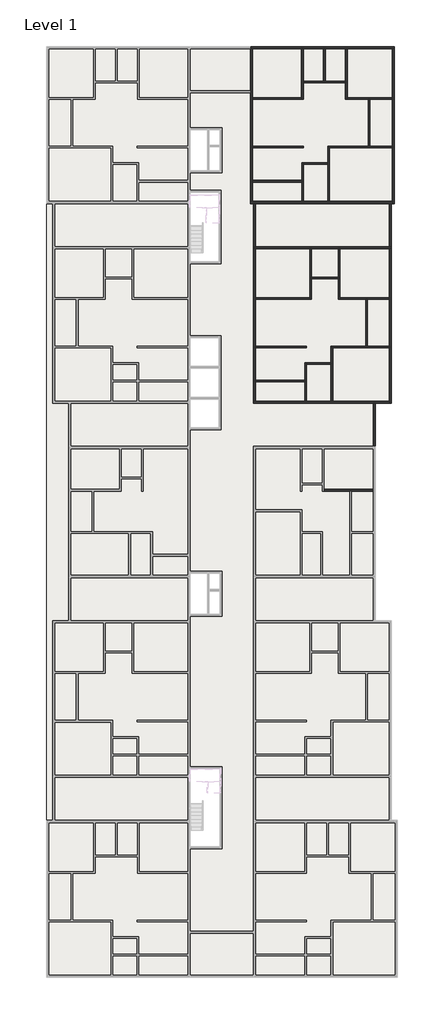
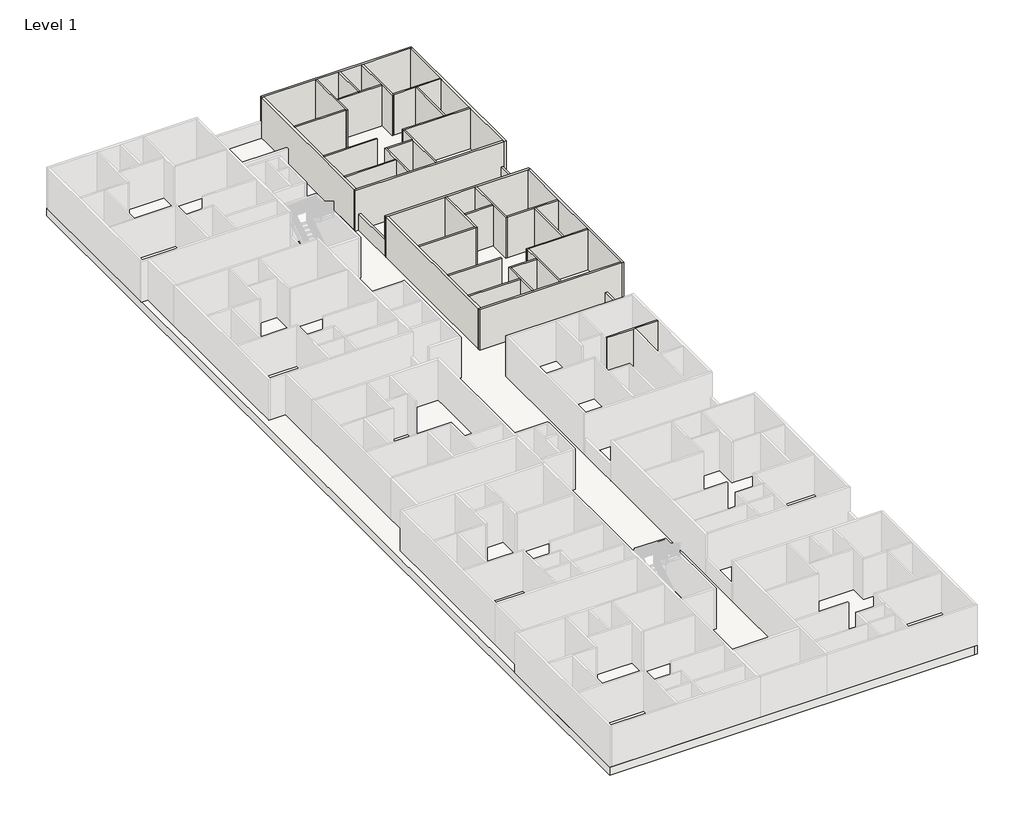
# One storey, part 4 of 8: 37 walls, 1 slab.
"""IFC4 building model written with IfcOpenShell, lengths in millimetres."""

from ifc_helpers import new_model, si_unit, frame, origin, place, context, project, spatial, polyline, outline, extrude, faceted_brep, element, save

model = new_model("IFC4")

# Units and contexts
model_context = context("Model", 3, world=origin())
ifc_project = project(units=[si_unit("LENGTHUNIT", "METRE", prefix="MILLI")], contexts=[model_context])

# Site, building, storey
site = spatial("IfcSite", under=ifc_project)
building = spatial("IfcBuilding", under=site)
storey = spatial("IfcBuildingStorey", under=building, Name="Level 1", Elevation=25234.6172466)

# Slab
placement = place(None, origin())
element("IfcSlab", 1, ObjectType="FLOOR", at=placement, inside=storey, context=model_context, shape_type="SweptSolid", body=[
    extrude(outline(polyline([(-14323.5415084, 35183.5216096), (11584.5443719, 35183.5216096), (11584.5443719, 23499.5216096), (11360.9214687, 23499.5216096), (11360.9214687, 8615.1216096), (10173.4714687, 8615.1216096), (10173.4714687, -7538.7344126), (11360.9214687, -7538.7344126), (11360.9214687, -22423.1344126), (11813.0584916, -22423.1344126), (11813.0584916, -34107.1344126), (11584.5443719, -34107.1344126), (-14323.5415084, -34107.1344126), (-14323.5415084, 35183.5216096)]), holes=[polyline([(-3617.4415084, 29152.4900967), (-3617.4415084, 25799.6900967), (-1255.2415084, 25799.6900967), (-1255.2415084, 29152.4900967), (-3617.4415084, 29152.4900967)]), polyline([(-3617.4415084, 24490.1216096), (-3617.4415084, 19003.7216096), (-1331.4415084, 19003.7216096), (-1331.4415084, 24490.1216096), (-3617.4415084, 24490.1216096)]), polyline([(-3617.4415084, 13669.6303368), (-3617.4415084, 6659.2303368), (-1331.4415084, 6659.2303368), (-1331.4415084, 13669.6303368), (-3617.4415084, 13669.6303368)]), polyline([(-3617.4415084, -3882.2751812), (-3617.4415084, -7235.0751812), (-1255.2415084, -7235.0751812), (-1255.2415084, -3882.2751812), (-3617.4415084, -3882.2751812)]), polyline([(-3617.4415084, -18429.9851539), (-3617.4415084, -24525.9851539), (-1229.8415084, -24525.9851539), (-1229.8415084, -18429.9851539), (-3617.4415084, -18429.9851539)])]), frame((0.0, 0.0, 24625.0172466), z_axis=(0.0, 0.0, 1.0), x_axis=(1.0, 0.0, 0.0)), (0.0, 0.0, 1.0), 609.6),
])

# Walls
element("IfcWall", 2, ObjectType="4.5\"", at=placement, inside=storey, context=model_context, shape_type="Brep", body=[
    faceted_brep([(6363.4714687, 2100.0216096, 25234.6172466), (8282.4584916, 2100.0216096, 25234.6172466), (8396.7584916, 2100.0216096, 25234.6172466), (10021.0714687, 2100.0216096, 25234.6172466), (10021.0714687, 2100.0216096, 28282.6172466), (8396.7584916, 2100.0216096, 28282.6172466), (8282.4584916, 2100.0216096, 28282.6172466), (6363.4714687, 2100.0216096, 28282.6172466), (6363.4714687, 2214.3216096, 25234.6172466), (6363.4714687, 2214.3216096, 28282.6172466), (10021.0714687, 2214.3216096, 28282.6172466), (10021.0714687, 2214.3216096, 25234.6172466)], [[[0, 1, 2, 3, 4, 5, 6, 7]], [[8, 9, 10, 11]], [[3, 2, 1, 0, 8, 11]], [[0, 7, 9, 8]], [[4, 3, 11, 10]], [[7, 6, 5, 4, 10, 9]]]),
])
element("IfcWall", 3, ObjectType="4.5\"", at=placement, inside=storey, context=model_context, shape_type="Brep", body=[
    faceted_brep([(5315.7214687, 20146.7216096, 25234.6172466), (5315.7214687, 16489.1216096, 25234.6172466), (5315.7214687, 16374.8216096, 25234.6172466), (5315.7214687, 16374.8216096, 28282.6172466), (5315.7214687, 16489.1216096, 28282.6172466), (5315.7214687, 20146.7216096, 28282.6172466), (5430.0214687, 20146.7216096, 25234.6172466), (5430.0214687, 20146.7216096, 28282.6172466), (5430.0214687, 18013.1216096, 28282.6172466), (5430.0214687, 17898.8216096, 28282.6172466), (5430.0214687, 16374.8216096, 28282.6172466), (5430.0214687, 16374.8216096, 25234.6172466), (5430.0214687, 17898.8216096, 25234.6172466), (5430.0214687, 18013.1216096, 25234.6172466)], [[[0, 1, 2, 3, 4, 5]], [[6, 7, 8, 9, 10, 11, 12, 13]], [[2, 1, 0, 6, 13, 12, 11]], [[0, 5, 7, 6]], [[3, 2, 11, 10]], [[5, 4, 3, 10, 9, 8, 7]]]),
])
element("IfcWall", 4, ObjectType="4.5\"", at=placement, inside=storey, context=model_context, shape_type="SweptSolid", body=[
    extrude(outline(polyline([(1259.3584916, 16489.1216096), (5315.7214687, 16489.1216096), (5315.7214687, 16374.8216096), (1259.3584916, 16374.8216096), (1259.3584916, 16489.1216096)])), frame((0.0, 0.0, 25234.6172466), z_axis=(0.0, 0.0, 1.0), x_axis=(1.0, 0.0, 0.0)), (0.0, 0.0, 1.0), 3048.0),
])
element("IfcWall", 5, ObjectType="4.5\"", at=placement, inside=storey, context=model_context, shape_type="SweptSolid", body=[
    extrude(outline(polyline([(7436.6214687, 17898.8216096), (5430.0214687, 17898.8216096), (5430.0214687, 18013.1216096), (7436.6214687, 18013.1216096), (7436.6214687, 17898.8216096)])), frame((0.0, 0.0, 25234.6172466), z_axis=(0.0, 0.0, 1.0), x_axis=(1.0, 0.0, 0.0)), (0.0, 0.0, 1.0), 3048.0),
])
element("IfcWall", 6, ObjectType="4.5\"", at=placement, inside=storey, context=model_context, shape_type="Brep", body=[
    faceted_brep([(7436.6214687, 20146.7216096, 25234.6172466), (7436.6214687, 18013.1216096, 25234.6172466), (7436.6214687, 17898.8216096, 25234.6172466), (7436.6214687, 16374.8216096, 25234.6172466), (7436.6214687, 16374.8216096, 28282.6172466), (7436.6214687, 17898.8216096, 28282.6172466), (7436.6214687, 18013.1216096, 28282.6172466), (7436.6214687, 20146.7216096, 28282.6172466), (7550.9214687, 20146.7216096, 25234.6172466), (7550.9214687, 20146.7216096, 28282.6172466), (7550.9214687, 16489.1216096, 28282.6172466), (7550.9214687, 16374.8216096, 28282.6172466), (7550.9214687, 16374.8216096, 25234.6172466), (7550.9214687, 16489.1216096, 25234.6172466)], [[[0, 1, 2, 3, 4, 5, 6, 7]], [[8, 9, 10, 11, 12, 13]], [[3, 2, 1, 0, 8, 13, 12]], [[0, 7, 9, 8]], [[4, 3, 12, 11]], [[7, 6, 5, 4, 11, 10, 9]]]),
])
element("IfcWall", 7, ObjectType="4.5\"", at=placement, inside=storey, context=model_context, shape_type="Brep", body=[
    faceted_brep([(7550.9214687, 16374.8216096, 25234.6172466), (9469.9084916, 16374.8216096, 25234.6172466), (9584.2084916, 16374.8216096, 25234.6172466), (11208.5214687, 16374.8216096, 25234.6172466), (11208.5214687, 16374.8216096, 28282.6172466), (9584.2084916, 16374.8216096, 28282.6172466), (9469.9084916, 16374.8216096, 28282.6172466), (7550.9214687, 16374.8216096, 28282.6172466), (7550.9214687, 16489.1216096, 25234.6172466), (7550.9214687, 16489.1216096, 28282.6172466), (11208.5214687, 16489.1216096, 28282.6172466), (11208.5214687, 16489.1216096, 25234.6172466)], [[[0, 1, 2, 3, 4, 5, 6, 7]], [[8, 9, 10, 11]], [[3, 2, 1, 0, 8, 11]], [[0, 7, 9, 8]], [[4, 3, 11, 10]], [[7, 6, 5, 4, 10, 9]]]),
])
element("IfcWall", 8, ObjectType="4.5\"", at=placement, inside=storey, context=model_context, shape_type="SweptSolid", body=[
    extrude(outline(polyline([(9469.9084916, 12869.6216096), (9469.9084916, 16374.8216096), (9584.2084916, 16374.8216096), (9584.2084916, 12869.6216096), (9469.9084916, 12869.6216096)])), frame((0.0, 0.0, 25234.6172466), z_axis=(0.0, 0.0, 1.0), x_axis=(1.0, 0.0, 0.0)), (0.0, 0.0, 1.0), 3048.0),
])
element("IfcWall", 9, ObjectType="4.5\"", at=placement, inside=storey, context=model_context, shape_type="Brep", body=[
    faceted_brep([(11208.5214687, 12869.6216096, 25234.6172466), (9584.2084916, 12869.6216096, 25234.6172466), (9469.9084916, 12869.6216096, 25234.6172466), (6885.4584916, 12869.6216096, 25234.6172466), (6885.4584916, 12869.6216096, 28282.6172466), (9469.9084916, 12869.6216096, 28282.6172466), (9584.2084916, 12869.6216096, 28282.6172466), (11208.5214687, 12869.6216096, 28282.6172466), (11208.5214687, 12755.3216096, 25234.6172466), (11208.5214687, 12755.3216096, 28282.6172466), (6999.7584916, 12755.3216096, 28282.6172466), (6885.4584916, 12755.3216096, 28282.6172466), (6885.4584916, 12755.3216096, 25234.6172466), (6999.7584916, 12755.3216096, 25234.6172466)], [[[0, 1, 2, 3, 4, 5, 6, 7]], [[8, 9, 10, 11, 12, 13]], [[3, 2, 1, 0, 8, 13, 12]], [[0, 7, 9, 8]], [[4, 3, 12, 11]], [[7, 6, 5, 4, 11, 10, 9]]]),
])
element("IfcWall", 10, ObjectType="4.5\"", at=placement, inside=storey, context=model_context, shape_type="Brep", body=[
    faceted_brep([(6885.4584916, 12755.3216096, 25234.6172466), (6885.4584916, 11663.1216096, 25234.6172466), (6885.4584916, 11548.8216096, 25234.6172466), (6885.4584916, 8767.5216096, 25234.6172466), (6885.4584916, 8767.5216096, 28282.6172466), (6885.4584916, 11548.8216096, 28282.6172466), (6885.4584916, 11663.1216096, 28282.6172466), (6885.4584916, 12755.3216096, 28282.6172466), (6999.7584916, 12755.3216096, 25234.6172466), (6999.7584916, 12755.3216096, 28282.6172466), (6999.7584916, 8767.5216096, 28282.6172466), (6999.7584916, 8767.5216096, 25234.6172466)], [[[0, 1, 2, 3, 4, 5, 6, 7]], [[8, 9, 10, 11]], [[3, 2, 1, 0, 8, 11]], [[0, 7, 9, 8]], [[4, 3, 11, 10]], [[7, 6, 5, 4, 10, 9]]]),
])
element("IfcWall", 11, ObjectType="4.5\"", at=placement, inside=storey, context=model_context, shape_type="Brep", body=[
    faceted_brep([(5056.6584916, 8767.5216096, 25234.6172466), (5056.6584916, 11548.8216096, 25234.6172466), (5056.6584916, 11663.1216096, 25234.6172466), (5056.6584916, 11663.1216096, 28282.6172466), (5056.6584916, 11548.8216096, 28282.6172466), (5056.6584916, 8767.5216096, 28282.6172466), (4942.3584916, 8767.5216096, 25234.6172466), (4942.3584916, 8767.5216096, 28282.6172466), (4942.3584916, 10215.3216096, 28282.6172466), (4942.3584916, 10329.6216096, 28282.6172466), (4942.3584916, 11663.1216096, 28282.6172466), (4942.3584916, 11663.1216096, 25234.6172466), (4942.3584916, 10329.6216096, 25234.6172466), (4942.3584916, 10215.3216096, 25234.6172466)], [[[0, 1, 2, 3, 4, 5]], [[6, 7, 8, 9, 10, 11, 12, 13]], [[2, 1, 0, 6, 13, 12, 11]], [[0, 5, 7, 6]], [[3, 2, 11, 10]], [[5, 4, 3, 10, 9, 8, 7]]]),
])
element("IfcWall", 12, ObjectType="4.5\"", at=placement, inside=storey, context=model_context, shape_type="SweptSolid", body=[
    extrude(outline(polyline([(6885.4584916, 11548.8216096), (5056.6584916, 11548.8216096), (5056.6584916, 11663.1216096), (6885.4584916, 11663.1216096), (6885.4584916, 11548.8216096)])), frame((0.0, 0.0, 25234.6172466), z_axis=(0.0, 0.0, 1.0), x_axis=(1.0, 0.0, 0.0)), (0.0, 0.0, 1.0), 3048.0),
])
element("IfcWall", 13, ObjectType="4.5\"", at=placement, inside=storey, context=model_context, shape_type="SweptSolid", body=[
    extrude(outline(polyline([(4942.3584916, 10215.3216096), (1259.3584916, 10215.3216096), (1259.3584916, 10329.6216096), (4942.3584916, 10329.6216096), (4942.3584916, 10215.3216096)])), frame((0.0, 0.0, 25234.6172466), z_axis=(0.0, 0.0, 1.0), x_axis=(1.0, 0.0, 0.0)), (0.0, 0.0, 1.0), 3048.0),
])
element("IfcWall", 14, ObjectType="4.5\"", at=placement, inside=storey, context=model_context, shape_type="SweptSolid", body=[
    extrude(outline(polyline([(5056.6584916, 12755.3216096), (1259.3584916, 12755.3216096), (1259.3584916, 12869.6216096), (5056.6584916, 12869.6216096), (5056.6584916, 12755.3216096)])), frame((0.0, 0.0, 25234.6172466), z_axis=(0.0, 0.0, 1.0), x_axis=(1.0, 0.0, 0.0)), (0.0, 0.0, 1.0), 3048.0),
])
element("IfcWall", 15, ObjectType="4.5\"", at=placement, inside=storey, context=model_context, shape_type="Brep", body=[
    faceted_brep([(4688.4443719, 35031.1216096, 25234.6172466), (4688.4443719, 31373.5216096, 25234.6172466), (4688.4443719, 31259.2216096, 25234.6172466), (4688.4443719, 31259.2216096, 28282.6172466), (4688.4443719, 31373.5216096, 28282.6172466), (4688.4443719, 35031.1216096, 28282.6172466), (4802.7443719, 35031.1216096, 25234.6172466), (4802.7443719, 35031.1216096, 28282.6172466), (4802.7443719, 32592.7216096, 28282.6172466), (4802.7443719, 32478.4216096, 28282.6172466), (4802.7443719, 31259.2216096, 28282.6172466), (4802.7443719, 31259.2216096, 25234.6172466), (4802.7443719, 32478.4216096, 25234.6172466), (4802.7443719, 32592.7216096, 25234.6172466)], [[[0, 1, 2, 3, 4, 5]], [[6, 7, 8, 9, 10, 11, 12, 13]], [[2, 1, 0, 6, 13, 12, 11]], [[0, 5, 7, 6]], [[3, 2, 11, 10]], [[5, 4, 3, 10, 9, 8, 7]]]),
])
element("IfcWall", 16, ObjectType="4.5\"", at=placement, inside=storey, context=model_context, shape_type="SweptSolid", body=[
    extrude(outline(polyline([(1030.8443719, 31373.5216096), (4688.4443719, 31373.5216096), (4688.4443719, 31259.2216096), (1030.8443719, 31259.2216096), (1030.8443719, 31373.5216096)])), frame((0.0, 0.0, 25234.6172466), z_axis=(0.0, 0.0, 1.0), x_axis=(1.0, 0.0, 0.0)), (0.0, 0.0, 1.0), 3048.0),
])
element("IfcWall", 17, ObjectType="4.5\"", at=placement, inside=storey, context=model_context, shape_type="Brep", body=[
    faceted_brep([(4802.7443719, 32478.4216096, 25234.6172466), (7965.0443719, 32478.4216096, 25234.6172466), (7965.0443719, 32478.4216096, 28282.6172466), (4802.7443719, 32478.4216096, 28282.6172466), (4802.7443719, 32592.7216096, 25234.6172466), (4802.7443719, 32592.7216096, 28282.6172466), (6326.7443719, 32592.7216096, 28282.6172466), (6441.0443719, 32592.7216096, 28282.6172466), (7965.0443719, 32592.7216096, 28282.6172466), (7965.0443719, 32592.7216096, 25234.6172466), (6441.0443719, 32592.7216096, 25234.6172466), (6326.7443719, 32592.7216096, 25234.6172466)], [[[0, 1, 2, 3]], [[4, 5, 6, 7, 8, 9, 10, 11]], [[1, 0, 4, 11, 10, 9]], [[0, 3, 5, 4]], [[2, 1, 9, 8]], [[3, 2, 8, 7, 6, 5]]]),
])
element("IfcWall", 18, ObjectType="4.5\"", at=placement, inside=storey, context=model_context, shape_type="SweptSolid", body=[
    extrude(outline(polyline([(6326.7443719, 32592.7216096), (6326.7443719, 35031.1216096), (6441.0443719, 35031.1216096), (6441.0443719, 32592.7216096), (6326.7443719, 32592.7216096)])), frame((0.0, 0.0, 25234.6172466), z_axis=(0.0, 0.0, 1.0), x_axis=(1.0, 0.0, 0.0)), (0.0, 0.0, 1.0), 3048.0),
])
element("IfcWall", 19, ObjectType="4.5\"", at=placement, inside=storey, context=model_context, shape_type="Brep", body=[
    faceted_brep([(7965.0443719, 35031.1216096, 25234.6172466), (7965.0443719, 32592.7216096, 25234.6172466), (7965.0443719, 32478.4216096, 25234.6172466), (7965.0443719, 31259.2216096, 25234.6172466), (7965.0443719, 31259.2216096, 28282.6172466), (7965.0443719, 32478.4216096, 28282.6172466), (7965.0443719, 32592.7216096, 28282.6172466), (7965.0443719, 35031.1216096, 28282.6172466), (8079.3443719, 35031.1216096, 25234.6172466), (8079.3443719, 35031.1216096, 28282.6172466), (8079.3443719, 31373.5216096, 28282.6172466), (8079.3443719, 31259.2216096, 28282.6172466), (8079.3443719, 31259.2216096, 25234.6172466), (8079.3443719, 31373.5216096, 25234.6172466)], [[[0, 1, 2, 3, 4, 5, 6, 7]], [[8, 9, 10, 11, 12, 13]], [[3, 2, 1, 0, 8, 13, 12]], [[0, 7, 9, 8]], [[4, 3, 12, 11]], [[7, 6, 5, 4, 11, 10, 9]]]),
])
element("IfcWall", 20, ObjectType="4.5\"", at=placement, inside=storey, context=model_context, shape_type="Brep", body=[
    faceted_brep([(8079.3443719, 31259.2216096, 25234.6172466), (9641.4443719, 31259.2216096, 25234.6172466), (9755.7443719, 31259.2216096, 25234.6172466), (11432.1443719, 31259.2216096, 25234.6172466), (11432.1443719, 31259.2216096, 28282.6172466), (9755.7443719, 31259.2216096, 28282.6172466), (9641.4443719, 31259.2216096, 28282.6172466), (8079.3443719, 31259.2216096, 28282.6172466), (8079.3443719, 31373.5216096, 25234.6172466), (8079.3443719, 31373.5216096, 28282.6172466), (11432.1443719, 31373.5216096, 28282.6172466), (11432.1443719, 31373.5216096, 25234.6172466)], [[[0, 1, 2, 3, 4, 5, 6, 7]], [[8, 9, 10, 11]], [[3, 2, 1, 0, 8, 11]], [[0, 7, 9, 8]], [[4, 3, 11, 10]], [[7, 6, 5, 4, 10, 9]]]),
])
element("IfcWall", 21, ObjectType="4.5\"", at=placement, inside=storey, context=model_context, shape_type="SweptSolid", body=[
    extrude(outline(polyline([(9641.4443719, 27754.0216096), (9641.4443719, 31259.2216096), (9755.7443719, 31259.2216096), (9755.7443719, 27754.0216096), (9641.4443719, 27754.0216096)])), frame((0.0, 0.0, 25234.6172466), z_axis=(0.0, 0.0, 1.0), x_axis=(1.0, 0.0, 0.0)), (0.0, 0.0, 1.0), 3048.0),
])
element("IfcWall", 22, ObjectType="4.5\"", at=placement, inside=storey, context=model_context, shape_type="Brep", body=[
    faceted_brep([(11432.1443719, 27754.0216096, 25234.6172466), (9755.7443719, 27754.0216096, 25234.6172466), (9641.4443719, 27754.0216096, 25234.6172466), (6656.9443719, 27754.0216096, 25234.6172466), (6656.9443719, 27754.0216096, 28282.6172466), (9641.4443719, 27754.0216096, 28282.6172466), (9755.7443719, 27754.0216096, 28282.6172466), (11432.1443719, 27754.0216096, 28282.6172466), (11432.1443719, 27639.7216096, 25234.6172466), (11432.1443719, 27639.7216096, 28282.6172466), (6771.2443719, 27639.7216096, 28282.6172466), (6656.9443719, 27639.7216096, 28282.6172466), (6656.9443719, 27639.7216096, 25234.6172466), (6771.2443719, 27639.7216096, 25234.6172466)], [[[0, 1, 2, 3, 4, 5, 6, 7]], [[8, 9, 10, 11, 12, 13]], [[3, 2, 1, 0, 8, 13, 12]], [[0, 7, 9, 8]], [[4, 3, 12, 11]], [[7, 6, 5, 4, 11, 10, 9]]]),
])
element("IfcWall", 23, ObjectType="4.5\"", at=placement, inside=storey, context=model_context, shape_type="Brep", body=[
    faceted_brep([(6656.9443719, 27639.7216096, 25234.6172466), (6656.9443719, 26547.5216096, 25234.6172466), (6656.9443719, 26433.2216096, 25234.6172466), (6656.9443719, 23651.9216096, 25234.6172466), (6656.9443719, 23651.9216096, 28282.6172466), (6656.9443719, 26433.2216096, 28282.6172466), (6656.9443719, 26547.5216096, 28282.6172466), (6656.9443719, 27639.7216096, 28282.6172466), (6771.2443719, 27639.7216096, 25234.6172466), (6771.2443719, 27639.7216096, 28282.6172466), (6771.2443719, 23651.9216096, 28282.6172466), (6771.2443719, 23651.9216096, 25234.6172466)], [[[0, 1, 2, 3, 4, 5, 6, 7]], [[8, 9, 10, 11]], [[3, 2, 1, 0, 8, 11]], [[0, 7, 9, 8]], [[4, 3, 11, 10]], [[7, 6, 5, 4, 10, 9]]]),
])
element("IfcWall", 24, ObjectType="4.5\"", at=placement, inside=storey, context=model_context, shape_type="SweptSolid", body=[
    extrude(outline(polyline([(4713.8443719, 25099.7216096), (1030.8443719, 25099.7216096), (1030.8443719, 25214.0216096), (4713.8443719, 25214.0216096), (4713.8443719, 25099.7216096)])), frame((0.0, 0.0, 25234.6172466), z_axis=(0.0, 0.0, 1.0), x_axis=(1.0, 0.0, 0.0)), (0.0, 0.0, 1.0), 3048.0),
])
element("IfcWall", 25, ObjectType="4.5\"", at=placement, inside=storey, context=model_context, shape_type="Brep", body=[
    faceted_brep([(4828.1443719, 23651.9216096, 25234.6172466), (4828.1443719, 26433.2216096, 25234.6172466), (4828.1443719, 26547.5216096, 25234.6172466), (4828.1443719, 26547.5216096, 28282.6172466), (4828.1443719, 26433.2216096, 28282.6172466), (4828.1443719, 23651.9216096, 28282.6172466), (4713.8443719, 23651.9216096, 25234.6172466), (4713.8443719, 23651.9216096, 28282.6172466), (4713.8443719, 25099.7216096, 28282.6172466), (4713.8443719, 25214.0216096, 28282.6172466), (4713.8443719, 26547.5216096, 28282.6172466), (4713.8443719, 26547.5216096, 25234.6172466), (4713.8443719, 25214.0216096, 25234.6172466), (4713.8443719, 25099.7216096, 25234.6172466)], [[[0, 1, 2, 3, 4, 5]], [[6, 7, 8, 9, 10, 11, 12, 13]], [[2, 1, 0, 6, 13, 12, 11]], [[0, 5, 7, 6]], [[3, 2, 11, 10]], [[5, 4, 3, 10, 9, 8, 7]]]),
])
element("IfcWall", 26, ObjectType="4.5\"", at=placement, inside=storey, context=model_context, shape_type="SweptSolid", body=[
    extrude(outline(polyline([(6656.9443719, 26433.2216096), (4828.1443719, 26433.2216096), (4828.1443719, 26547.5216096), (6656.9443719, 26547.5216096), (6656.9443719, 26433.2216096)])), frame((0.0, 0.0, 25234.6172466), z_axis=(0.0, 0.0, 1.0), x_axis=(1.0, 0.0, 0.0)), (0.0, 0.0, 1.0), 3048.0),
])
element("IfcWall", 27, ObjectType="4.5\"", at=placement, inside=storey, context=model_context, shape_type="SweptSolid", body=[
    extrude(outline(polyline([(4828.1443719, 27639.7216096), (1030.8443719, 27639.7216096), (1030.8443719, 27754.0216096), (4828.1443719, 27754.0216096), (4828.1443719, 27639.7216096)])), frame((0.0, 0.0, 25234.6172466), z_axis=(0.0, 0.0, 1.0), x_axis=(1.0, 0.0, 0.0)), (0.0, 0.0, 1.0), 3048.0),
])
element("IfcWall", 28, ObjectType="6\"", at=placement, inside=storey, context=model_context, shape_type="Brep", body=[
    faceted_brep([(1106.9584916, 20146.7216096, 28282.6172466), (1106.9584916, 20146.7216096, 25234.6172466), (1259.3584916, 20146.7216096, 25234.6172466), (5315.7214687, 20146.7216096, 25234.6172466), (5430.0214687, 20146.7216096, 25234.6172466), (7436.6214687, 20146.7216096, 25234.6172466), (7550.9214687, 20146.7216096, 25234.6172466), (11208.5214687, 20146.7216096, 25234.6172466), (11360.9214687, 20146.7216096, 25234.6172466), (11360.9214687, 20146.7216096, 28282.6172466), (11208.5214687, 20146.7216096, 28282.6172466), (7550.9214687, 20146.7216096, 28282.6172466), (7436.6214687, 20146.7216096, 28282.6172466), (5430.0214687, 20146.7216096, 28282.6172466), (5315.7214687, 20146.7216096, 28282.6172466), (1259.3584916, 20146.7216096, 28282.6172466), (1106.9584916, 20299.1216096, 25234.6172466), (1106.9584916, 20299.1216096, 26453.8172466), (1106.9584916, 20299.1216096, 28282.6172466), (11360.9214687, 20299.1216096, 28282.6172466), (11360.9214687, 20299.1216096, 26453.8172466), (11360.9214687, 20299.1216096, 25234.6172466), (11208.5214687, 20299.1216096, 25234.6172466), (1259.3584916, 20299.1216096, 25234.6172466)], [[[0, 1, 2, 3, 4, 5, 6, 7, 8, 9, 10, 11, 12, 13, 14, 15]], [[16, 17, 18, 19, 20, 21, 22, 23]], [[8, 7, 6, 5, 4, 3, 2, 1, 16, 23, 22, 21]], [[0, 18, 17, 16, 1]], [[8, 21, 20, 19, 9]], [[0, 15, 14, 13, 12, 11, 10, 9, 19, 18]]]),
])
element("IfcWall", 29, ObjectType="6\"", at=placement, inside=storey, context=model_context, shape_type="Brep", body=[
    faceted_brep([(11208.5214687, 20146.7216096, 28282.6172466), (11208.5214687, 20146.7216096, 25234.6172466), (11208.5214687, 16489.1216096, 25234.6172466), (11208.5214687, 16374.8216096, 25234.6172466), (11208.5214687, 12869.6216096, 25234.6172466), (11208.5214687, 12755.3216096, 25234.6172466), (11208.5214687, 8767.5216096, 25234.6172466), (11208.5214687, 8615.1216096, 25234.6172466), (11208.5214687, 8615.1216096, 28282.6172466), (11208.5214687, 8767.5216096, 28282.6172466), (11208.5214687, 12755.3216096, 28282.6172466), (11208.5214687, 12869.6216096, 28282.6172466), (11208.5214687, 16374.8216096, 28282.6172466), (11208.5214687, 16489.1216096, 28282.6172466), (11360.9214687, 20146.7216096, 25234.6172466), (11360.9214687, 20146.7216096, 28282.6172466), (11360.9214687, 8615.1216096, 28282.6172466), (11360.9214687, 8615.1216096, 25234.6172466)], [[[0, 1, 2, 3, 4, 5, 6, 7, 8, 9, 10, 11, 12, 13]], [[14, 15, 16, 17]], [[7, 6, 5, 4, 3, 2, 1, 14, 17]], [[8, 7, 17, 16]], [[0, 15, 14, 1]], [[0, 13, 12, 11, 10, 9, 8, 16, 15]]]),
])
element("IfcWall", 30, ObjectType="6\"", at=placement, inside=storey, context=model_context, shape_type="Brep", body=[
    faceted_brep([(11208.5214687, 8767.5216096, 25234.6172466), (6999.7584916, 8767.5216096, 25234.6172466), (6885.4584916, 8767.5216096, 25234.6172466), (5056.6584916, 8767.5216096, 25234.6172466), (4942.3584916, 8767.5216096, 25234.6172466), (1259.3584916, 8767.5216096, 25234.6172466), (1106.9584916, 8767.5216096, 25234.6172466), (1106.9584916, 8767.5216096, 28282.6172466), (1259.3584916, 8767.5216096, 28282.6172466), (4942.3584916, 8767.5216096, 28282.6172466), (5056.6584916, 8767.5216096, 28282.6172466), (6885.4584916, 8767.5216096, 28282.6172466), (6999.7584916, 8767.5216096, 28282.6172466), (11208.5214687, 8767.5216096, 28282.6172466), (11208.5214687, 8615.1216096, 25234.6172466), (11208.5214687, 8615.1216096, 28282.6172466), (1106.9584916, 8615.1216096, 28282.6172466), (1106.9584916, 8615.1216096, 25234.6172466), (10021.0714687, 8615.1216096, 25234.6172466), (10173.4714687, 8615.1216096, 25234.6172466)], [[[0, 1, 2, 3, 4, 5, 6, 7, 8, 9, 10, 11, 12, 13]], [[14, 15, 16, 17, 18, 19]], [[6, 5, 4, 3, 2, 1, 0, 14, 19, 18, 17]], [[0, 13, 15, 14]], [[7, 6, 17, 16]], [[13, 12, 11, 10, 9, 8, 7, 16, 15]]]),
])
element("IfcWall", 31, ObjectType="6\"", at=placement, inside=storey, context=model_context, shape_type="Brep", body=[
    faceted_brep([(1259.3584916, 8767.5216096, 25234.6172466), (1259.3584916, 10215.3216096, 25234.6172466), (1259.3584916, 10329.6216096, 25234.6172466), (1259.3584916, 12755.3216096, 25234.6172466), (1259.3584916, 12869.6216096, 25234.6172466), (1259.3584916, 16374.8216096, 25234.6172466), (1259.3584916, 16489.1216096, 25234.6172466), (1259.3584916, 20146.7216096, 25234.6172466), (1259.3584916, 20146.7216096, 28282.6172466), (1259.3584916, 16489.1216096, 28282.6172466), (1259.3584916, 16374.8216096, 28282.6172466), (1259.3584916, 12869.6216096, 28282.6172466), (1259.3584916, 12755.3216096, 28282.6172466), (1259.3584916, 10329.6216096, 28282.6172466), (1259.3584916, 10215.3216096, 28282.6172466), (1259.3584916, 8767.5216096, 28282.6172466), (1106.9584916, 8767.5216096, 25234.6172466), (1106.9584916, 8767.5216096, 28282.6172466), (1106.9584916, 20146.7216096, 28282.6172466), (1106.9584916, 20146.7216096, 25234.6172466)], [[[0, 1, 2, 3, 4, 5, 6, 7, 8, 9, 10, 11, 12, 13, 14, 15]], [[16, 17, 18, 19]], [[7, 6, 5, 4, 3, 2, 1, 0, 16, 19]], [[0, 15, 17, 16]], [[7, 19, 18, 8]], [[15, 14, 13, 12, 11, 10, 9, 8, 18, 17]]]),
])
element("IfcWall", 32, ObjectType="6\"", at=placement, inside=storey, context=model_context, shape_type="Brep", body=[
    faceted_brep([(878.4443719, 35031.1216096, 28282.6172466), (878.4443719, 35031.1216096, 25234.6172466), (1030.8443719, 35031.1216096, 25234.6172466), (4688.4443719, 35031.1216096, 25234.6172466), (4802.7443719, 35031.1216096, 25234.6172466), (6326.7443719, 35031.1216096, 25234.6172466), (6441.0443719, 35031.1216096, 25234.6172466), (7965.0443719, 35031.1216096, 25234.6172466), (8079.3443719, 35031.1216096, 25234.6172466), (11432.1443719, 35031.1216096, 25234.6172466), (11584.5443719, 35031.1216096, 25234.6172466), (11584.5443719, 35031.1216096, 28282.6172466), (11432.1443719, 35031.1216096, 28282.6172466), (8079.3443719, 35031.1216096, 28282.6172466), (7965.0443719, 35031.1216096, 28282.6172466), (6441.0443719, 35031.1216096, 28282.6172466), (6326.7443719, 35031.1216096, 28282.6172466), (4802.7443719, 35031.1216096, 28282.6172466), (4688.4443719, 35031.1216096, 28282.6172466), (1030.8443719, 35031.1216096, 28282.6172466), (878.4443719, 35183.5216096, 25234.6172466), (878.4443719, 35183.5216096, 28282.6172466), (11584.5443719, 35183.5216096, 28282.6172466), (11584.5443719, 35183.5216096, 25234.6172466)], [[[0, 1, 2, 3, 4, 5, 6, 7, 8, 9, 10, 11, 12, 13, 14, 15, 16, 17, 18, 19]], [[20, 21, 22, 23]], [[10, 9, 8, 7, 6, 5, 4, 3, 2, 1, 20, 23]], [[11, 10, 23, 22]], [[0, 21, 20, 1]], [[0, 19, 18, 17, 16, 15, 14, 13, 12, 11, 22, 21]]]),
])
element("IfcWall", 33, ObjectType="6\"", at=placement, inside=storey, context=model_context, shape_type="Brep", body=[
    faceted_brep([(11432.1443719, 35031.1216096, 25234.6172466), (11432.1443719, 31373.5216096, 25234.6172466), (11432.1443719, 31259.2216096, 25234.6172466), (11432.1443719, 27754.0216096, 25234.6172466), (11432.1443719, 27639.7216096, 25234.6172466), (11432.1443719, 23651.9216096, 25234.6172466), (11432.1443719, 23499.5216096, 25234.6172466), (11432.1443719, 23499.5216096, 28282.6172466), (11432.1443719, 23651.9216096, 28282.6172466), (11432.1443719, 27639.7216096, 28282.6172466), (11432.1443719, 27754.0216096, 28282.6172466), (11432.1443719, 31259.2216096, 28282.6172466), (11432.1443719, 31373.5216096, 28282.6172466), (11432.1443719, 35031.1216096, 28282.6172466), (11584.5443719, 35031.1216096, 25234.6172466), (11584.5443719, 35031.1216096, 28282.6172466), (11584.5443719, 23499.5216096, 28282.6172466), (11584.5443719, 23499.5216096, 25234.6172466)], [[[0, 1, 2, 3, 4, 5, 6, 7, 8, 9, 10, 11, 12, 13]], [[14, 15, 16, 17]], [[6, 5, 4, 3, 2, 1, 0, 14, 17]], [[0, 13, 15, 14]], [[7, 6, 17, 16]], [[13, 12, 11, 10, 9, 8, 7, 16, 15]]]),
])
element("IfcWall", 34, ObjectType="6\"", at=placement, inside=storey, context=model_context, shape_type="Brep", body=[
    faceted_brep([(11432.1443719, 23651.9216096, 25234.6172466), (6771.2443719, 23651.9216096, 25234.6172466), (6656.9443719, 23651.9216096, 25234.6172466), (4828.1443719, 23651.9216096, 25234.6172466), (4713.8443719, 23651.9216096, 25234.6172466), (1030.8443719, 23651.9216096, 25234.6172466), (878.4443719, 23651.9216096, 25234.6172466), (878.4443719, 23651.9216096, 28282.6172466), (1030.8443719, 23651.9216096, 28282.6172466), (4713.8443719, 23651.9216096, 28282.6172466), (4828.1443719, 23651.9216096, 28282.6172466), (6656.9443719, 23651.9216096, 28282.6172466), (6771.2443719, 23651.9216096, 28282.6172466), (11432.1443719, 23651.9216096, 28282.6172466), (11432.1443719, 23499.5216096, 25234.6172466), (11432.1443719, 23499.5216096, 28282.6172466), (878.4443719, 23499.5216096, 28282.6172466), (878.4443719, 23499.5216096, 25234.6172466), (1106.9584916, 23499.5216096, 25234.6172466), (1259.3584916, 23499.5216096, 25234.6172466), (11208.5214687, 23499.5216096, 25234.6172466), (11360.9214687, 23499.5216096, 25234.6172466)], [[[0, 1, 2, 3, 4, 5, 6, 7, 8, 9, 10, 11, 12, 13]], [[14, 15, 16, 17, 18, 19, 20, 21]], [[6, 5, 4, 3, 2, 1, 0, 14, 21, 20, 19, 18, 17]], [[0, 13, 15, 14]], [[7, 6, 17, 16]], [[13, 12, 11, 10, 9, 8, 7, 16, 15]]]),
])
element("IfcWall", 35, ObjectType="6\"", at=placement, inside=storey, context=model_context, shape_type="Brep", body=[
    faceted_brep([(1030.8443719, 23651.9216096, 25234.6172466), (1030.8443719, 25099.7216096, 25234.6172466), (1030.8443719, 25214.0216096, 25234.6172466), (1030.8443719, 27639.7216096, 25234.6172466), (1030.8443719, 27754.0216096, 25234.6172466), (1030.8443719, 31259.2216096, 25234.6172466), (1030.8443719, 31373.5216096, 25234.6172466), (1030.8443719, 35031.1216096, 25234.6172466), (1030.8443719, 35031.1216096, 28282.6172466), (1030.8443719, 31373.5216096, 28282.6172466), (1030.8443719, 31259.2216096, 28282.6172466), (1030.8443719, 27754.0216096, 28282.6172466), (1030.8443719, 27639.7216096, 28282.6172466), (1030.8443719, 25214.0216096, 28282.6172466), (1030.8443719, 25099.7216096, 28282.6172466), (1030.8443719, 23651.9216096, 28282.6172466), (878.4443719, 23651.9216096, 25234.6172466), (878.4443719, 23651.9216096, 28282.6172466), (878.4443719, 35031.1216096, 28282.6172466), (878.4443719, 35031.1216096, 25234.6172466), (878.4443719, 31897.3197155, 25234.6172466), (878.4443719, 31744.9197155, 25234.6172466)], [[[0, 1, 2, 3, 4, 5, 6, 7, 8, 9, 10, 11, 12, 13, 14, 15]], [[16, 17, 18, 19, 20, 21]], [[7, 6, 5, 4, 3, 2, 1, 0, 16, 21, 20, 19]], [[0, 15, 17, 16]], [[7, 19, 18, 8]], [[15, 14, 13, 12, 11, 10, 9, 8, 18, 17]]]),
])
element("IfcWall", 36, ObjectType="6\" 2", at=placement, inside=storey, context=model_context, shape_type="SweptSolid", body=[
    extrude(outline(polyline([(1106.9584916, 20299.1216096), (1106.9584916, 23499.5216096), (1259.3584916, 23499.5216096), (1259.3584916, 20299.1216096), (1106.9584916, 20299.1216096)])), frame((0.0, 0.0, 25234.6172466), z_axis=(0.0, 0.0, 1.0), x_axis=(1.0, 0.0, 0.0)), (0.0, 0.0, 1.0), 1219.2),
])
element("IfcWall", 37, ObjectType="6\" 2", at=placement, inside=storey, context=model_context, shape_type="SweptSolid", body=[
    extrude(outline(polyline([(11208.5214687, 20299.1216096), (11208.5214687, 23499.5216096), (11360.9214687, 23499.5216096), (11360.9214687, 20299.1216096), (11208.5214687, 20299.1216096)])), frame((0.0, 0.0, 25234.6172466), z_axis=(0.0, 0.0, 1.0), x_axis=(1.0, 0.0, 0.0)), (0.0, 0.0, 1.0), 1219.2),
])
element("IfcWall", 38, ObjectType="6\" 2", at=placement, inside=storey, context=model_context, shape_type="SweptSolid", body=[
    extrude(outline(polyline([(10021.0714687, 5414.7216096), (10021.0714687, 8615.1216096), (10173.4714687, 8615.1216096), (10173.4714687, 5414.7216096), (10021.0714687, 5414.7216096)])), frame((0.0, 0.0, 25234.6172466), z_axis=(0.0, 0.0, 1.0), x_axis=(1.0, 0.0, 0.0)), (0.0, 0.0, 1.0), 1219.2),
])

save(model, "model.ifc")

# Revit data of these elements
# Type "FLOOR"
#   Assembly Code = "B1010"
#   Function = 0
#   Layers, outside or top first: 2' - 0" "Tile, Porcelain, 4in" (function 1)
# Type "4.5\""
#   Assembly Code = "B2010"
#   Layers, outside or top first: 0' - 4 1/2" "WALLS" (function 1)
# Type "6\""
#   Assembly Code = "B2010"
#   Layers, outside or top first: 0' - 6" "WALLS" (function 1)
# Type "6\" 2"
#   Assembly Code = "B2010"
#   Layers, outside or top first: 0' - 6" "4'" (function 1)
# Element 1 (IfcSlab, "FLOOR")
#   built-in parameter 1001955 = 3.14159 (stored number, unit not read)
#   Height Offset From Level = 0' - 0"
#   Phase Created = New Construction
#   Materials on its faces: "Tile, Porcelain, 4in"
# Elements 2, 3, 4, 5, 6, 7, 8, 9, 10, 11, 12, 13, 14, 15, 16, 17, 18, 19, 20, 21, 22, 23, 24, 25, 26, 27 (IfcWall, "4.5\"")
#   Top Offset = 0' - 0"
#   Base Offset = 0' - 0"
#   Unconnected Height = 10' - 0"
#   wall height = 10' - 0"
#   Phase Created = New Construction
#   Base Constraint = Level 1
#   Materials on its faces: "WALLS"
# Elements 28, 29, 30, 31, 32, 33, 34, 35 (IfcWall, "6\"")
#   Top Offset = 0' - 0"
#   Base Offset = 0' - 0"
#   Unconnected Height = 10' - 0"
#   wall height = 10' - 0"
#   Phase Created = New Construction
#   Base Constraint = Level 1
#   Materials on its faces: "WALLS"
# Elements 36, 37, 38 (IfcWall, "6\" 2")
#   Top Offset = 0' - 0"
#   Base Offset = 0' - 0"
#   Unconnected Height = 4' - 0"
#   wall height = 4' - 0"
#   Phase Created = New Construction
#   Base Constraint = Level 1
#   Materials on its faces: "4'"
# Materials
#   "Tile, Porcelain, 4in": class "Generic", colour RGB 89 87 158, transparency 0, Description = "Porcelain tile, 4\", white", Cost = 0
#   "WALLS": class "Generic", colour RGB 120 120 120, transparency 0, Cost = 0
#   "4'": class "Generic", colour RGB 120 120 120, transparency 0, Cost = 0
